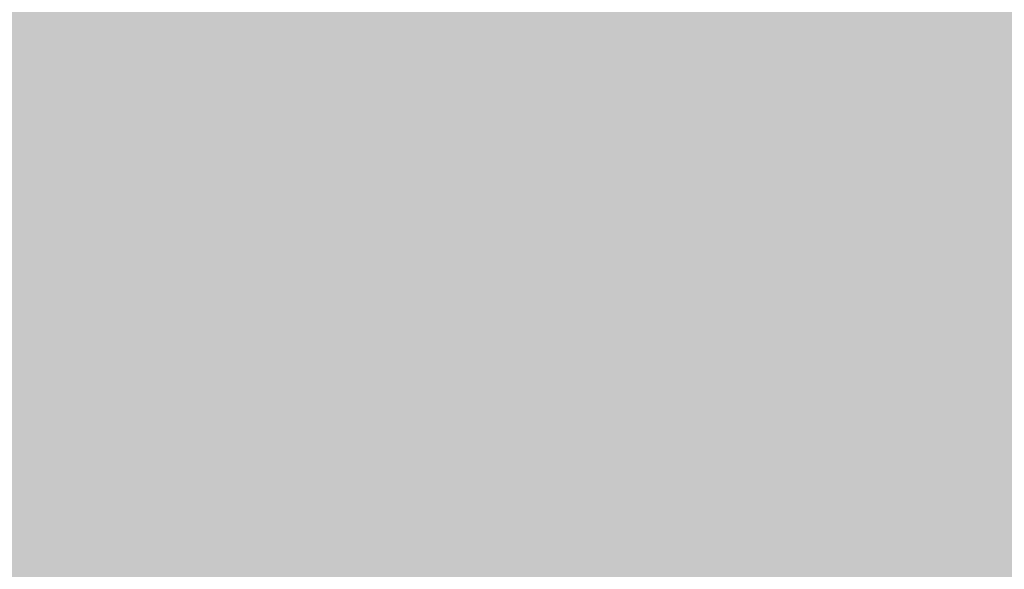
# Model space of a CAD drawing. Units: feet. Extents: x 3168 to 4724, y 827 to 1477.
# Tile 40 of 256: x 3270.273 to 3273.072, y 1096.781 to 1098.344. Entities that reach past the tile are written whole.
import ezdxf

# ---------------------------------------------------------------- set-up
doc = ezdxf.new("R2010")
doc.units = ezdxf.units.FT
doc.layers.add('A-ELEV-PATT', color=8, linetype='Continuous', lineweight=13)

msp = doc.modelspace()

# ---------------------------------------------------------------- hatches: boundary and pattern name
at = {"layer": 'A-ELEV-PATT'}
h = msp.add_hatch(color=256, dxfattribs=at)
h.dxf.hatch_style = 1
edge = h.paths.add_edge_path()
edge.add_ellipse((3552.9058, 979.2201), major_axis=(36.7449, 0), ratio=0.4848485, start_angle=0, end_angle=360)
edge = h.paths.add_edge_path()
edge.add_ellipse((3559.8916, 929.2523), major_axis=(36.7449, 0), ratio=0.4848485, start_angle=0, end_angle=360)
edge = h.paths.add_edge_path()
edge.add_line((3299.3168, 1198.6061), (3479.9167, 1198.6061))
edge.add_line((3479.9167, 1198.6061), (3479.9167, 1209.8686))
edge.add_spline(control_points=[(3479.9167, 1209.8686), (3464.3012, 1209.8686), (3448.6856, 1209.8686), (3410.9491, 1209.8686), (3388.8282, 1209.8686), (3355.6469, 1209.8686), (3344.5864, 1209.8686), (3327.9957, 1209.8686), (3322.4655, 1209.8686), (3314.1702, 1209.8686), (3311.4051, 1209.8686), (3307.2574, 1209.8686), (3305.8748, 1209.8686), (3303.801, 1209.8686), (3303.1097, 1209.8686), (3302.0728, 1209.8686), (3301.7272, 1209.8686), (3301.2087, 1209.8686), (3301.0359, 1209.8686), (3300.7767, 1209.8686), (3300.6903, 1209.8686), (3300.5606, 1209.8686), (3300.5174, 1209.8686), (3300.4526, 1209.8686), (3300.431, 1209.8686), (3300.3986, 1209.8686), (3300.3878, 1209.8686), (3300.3662, 1209.8686), (3300.3457, 1209.8686), (3300.3455, 1209.8686), (3300.3455, 1209.8686), (3300.3433, 1209.8686), (3300.3411, 1209.8686), (3300.3379, 1209.8686), (3300.3368, 1209.8686), (3300.3339, 1209.8686), (3300.3321, 1209.8686), (3300.3255, 1209.8686), (3300.3207, 1209.8686), (3300.3109, 1209.8686), (3300.306, 1209.8686), (3300.2905, 1209.8686), (3300.28, 1209.8686), (3300.2324, 1209.8688), (3300.1953, 1209.869), (3299.9511, 1209.8706), (3299.7448, 1209.8743), (3299.4368, 1209.8833), (3299.3344, 1209.8868), (3299.1811, 1209.8929), (3299.13, 1209.8951), (3298.6522, 1209.9168), (3298.2295, 1209.9457), (3297.6016, 1210.0024), (3297.3934, 1210.0235), (3297.0827, 1210.0583), (3296.9793, 1210.0705), (3296.293, 1210.1549), (3295.7181, 1210.2434), (3294.8687, 1210.3989), (3294.5877, 1210.4545), (3294.1693, 1210.5433), (3294.0304, 1210.5739), (3291.7071, 1211.1012), (3289.6536, 1211.8134), (3285.7763, 1213.564), (3283.9514, 1214.6035), (3280.5122, 1216.9801), (3278.8972, 1218.3176), (3276.3799, 1220.8295), (3275.416, 1221.9177), (3274.0393, 1223.7077), (3273.581, 1224.3495), (3273.1432, 1225.0163)], knot_values=[39.119033, 39.119033, 39.119033, 39.119033, 39.286353, 39.286353, 39.523379, 39.523379, 39.641892, 39.641892, 39.701148, 39.701148, 39.730777, 39.730777, 39.745591, 39.745591, 39.752998, 39.752998, 39.756701, 39.756701, 39.758553, 39.758553, 39.759479, 39.759479, 39.759942, 39.759942, 39.760173, 39.760173, 39.760289, 39.760289, 39.760405, 39.760405, 39.760463, 39.760463, 39.763389, 39.763389, 39.764851, 39.764851, 39.767304, 39.767304, 39.773825, 39.773825, 39.78057, 39.78057, 39.79477, 39.79477, 39.845194, 39.845194, 40.126715, 40.126715, 40.267476, 40.267476, 40.337856, 40.337856, 40.927023, 40.927023, 41.221606, 41.221606, 41.368898, 41.368898, 42.202622, 42.202622, 42.619485, 42.619485, 42.827916, 42.827916, 46.118323, 46.118323, 49.408731, 49.408731, 52.699139, 52.699139, 54.927489, 54.927489, 56.104228, 56.104228, 56.104228, 56.104228], weights=[1, 1, 1, 1, 1, 1, 1, 1, 1, 1, 1, 1, 1, 1, 1, 1, 1, 1, 1, 1, 1, 1, 1, 1, 1, 1, 1, 1, 1, 1, 1, 1, 1, 1, 1, 1, 1, 1, 1, 1, 1, 1, 1, 1, 1, 1, 1, 1, 1, 1, 1, 1, 1, 1, 1, 1, 1, 1, 1, 1, 1, 1, 1, 1, 1, 1, 1, 1, 1, 1, 1, 1, 1, 1], degree=3, periodic=0)
edge.add_line((3273.1432, 1225.0163), (3273.1432, 1099.0163))
edge.add_line((3273.1432, 1099.0163), (3299.3168, 1099.0163))
edge.add_line((3299.3168, 1099.0163), (3299.3168, 1198.6061))
edge = h.paths.add_edge_path()
edge.add_line((3304.7584, 1324.1581), (3479.9167, 1324.1581))
edge.add_line((3479.9167, 1324.1581), (3479.9167, 1335.7146))
edge.add_line((3479.9167, 1335.7146), (3269.1616, 1335.7146))
edge.add_spline(control_points=[(3269.1616, 1335.7146), (3264.0242, 1335.7146), (3258.3641, 1328.9582), (3259.2643, 1323.9003)], knot_values=[0, 0, 0, 0, 15.412191, 15.412191, 15.412191, 15.412191], degree=3, periodic=0)
edge.add_line((3259.2643, 1323.9003), (3265.5168, 1288.7691))
edge.add_line((3265.5168, 1288.7691), (3275.2651, 1261.5456))
edge.add_line((3275.2651, 1261.5456), (3304.7584, 1261.5456))
edge.add_line((3304.7584, 1261.5456), (3304.7584, 1324.1581))
h = msp.add_hatch(color=256, dxfattribs=at)
h.dxf.hatch_style = 1
h.paths.add_polyline_path([(3384.5252, 1099.0163), (3335.0292, 1099.0163), (3299.3168, 1099.0163), (3273.1432, 1099.0163), (3217.5654, 1099.0163), (3168.0693, 827.1163), (3335.0292, 827.1163)])

doc.saveas('drawing.dxf')
